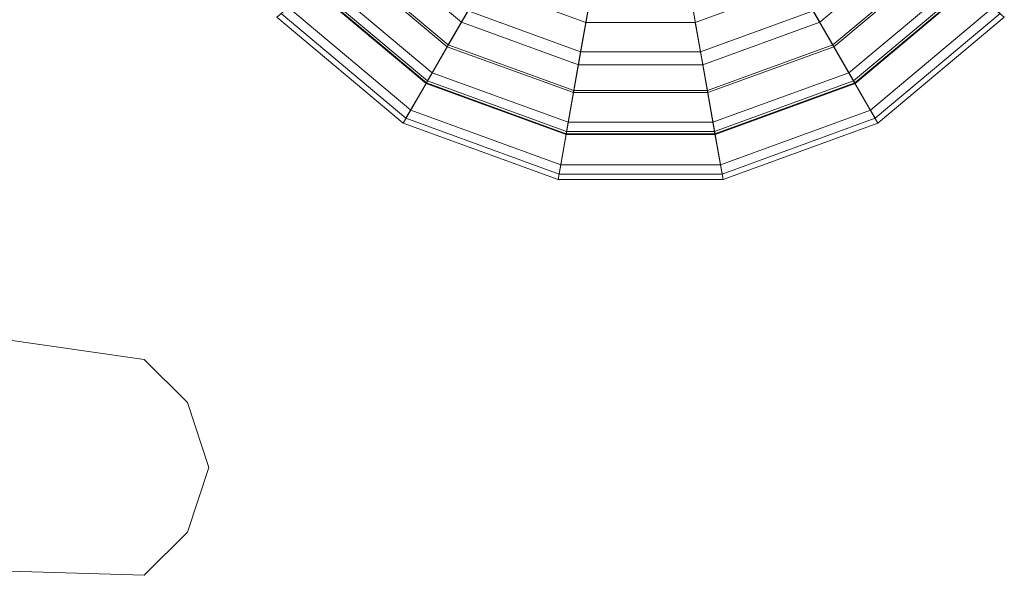
# Model space of a CAD drawing. Units: inches. Extents: x 375 to 1122, y 27 to 1069.
# Tile 20 of 155: x 717.492 to 720.301, y 270.778 to 272.362. Entities that reach past the tile are written whole.
import ezdxf

# ---------------------------------------------------------------- set-up
doc = ezdxf.new("R2010")
doc.units = ezdxf.units.IN
doc.layers.add('Furniture', color=30, linetype='Continuous', lineweight=18)

# ---------------------------------------------------------------- blocks, each defined once
blk = doc.blocks.new('A$C403C54AD')
for points in [[(1.855884, 0.874815, -0.031825), (1.826559, 0.857884, -0.028747), (1.826559, 0.857884, -0.028747), (1.848325, 0.883824, -0.031825)], [(1.853021, 0.873162, 0.131159), (1.855539, 0.874616, 0.117935), (1.848069, 0.883518, 0.117935), (1.8462, 0.881291, 0.131159)], [(1.853056, 0.873182, -0.028594), (1.855884, 0.874815, -0.031825), (1.848325, 0.883824, -0.031825), (1.846226, 0.881322, -0.028594)], [(1.855539, 0.874616, 0.117935), (1.854954, 0.874278, 0.089693), (1.847635, 0.883001, 0.089693), (1.848069, 0.883518, 0.117935)], [(1.854954, 0.874278, 0.089693), (1.850309, 0.871596, 0.071684), (1.844187, 0.878892, 0.071684), (1.847635, 0.883001, 0.089693)], [(1.838869, 0.864991, -0.02532), (1.853056, 0.873182, -0.028594), (1.846226, 0.881322, -0.028594), (1.835696, 0.868773, -0.02532)], [(1.847874, 0.87019, 0.073031), (1.852298, 0.872744, 0.090178), (1.845663, 0.880651, 0.090178), (1.84238, 0.876739, 0.073031)], [(1.848694, 0.870664, 0.140564), (1.853021, 0.873162, 0.131159), (1.8462, 0.881291, 0.131159), (1.842988, 0.877464, 0.140564)], [(1.852868, 0.873073, 0.117718), (1.850434, 0.871669, 0.130354), (1.84428, 0.879003, 0.130354), (1.846086, 0.881156, 0.117718)], [(1.852298, 0.872744, 0.090178), (1.852868, 0.873073, 0.117718), (1.846086, 0.881156, 0.117718), (1.845663, 0.880651, 0.090178)], [(1.850309, 0.871596, 0.071684), (1.844189, 0.868063, 0.061451), (1.839644, 0.873479, 0.061451), (1.844187, 0.878892, 0.071684)], [(1.850434, 0.871669, 0.130354), (1.846028, 0.869125, 0.140564), (1.84101, 0.875106, 0.140564), (1.84428, 0.879003, 0.130354)], [(1.846028, 0.869125, 0.140564), (1.848694, 0.870664, 0.140564), (1.842988, 0.877464, 0.140564), (1.84101, 0.875106, 0.140564)], [(1.859907, 0.863764, -0.031825), (1.826559, 0.857884, -0.028747), (1.826559, 0.857884, -0.028747), (1.855884, 0.874815, -0.031825)], [(1.858849, 0.863578, 0.089693), (1.853566, 0.862646, 0.071684), (1.850309, 0.871596, 0.071684), (1.854954, 0.874278, 0.089693)], [(1.856651, 0.86319, 0.131159), (1.859514, 0.863695, 0.117935), (1.855539, 0.874616, 0.117935), (1.853021, 0.873162, 0.131159)], [(1.85669, 0.863197, -0.028594), (1.859907, 0.863764, -0.031825), (1.855884, 0.874815, -0.031825), (1.853056, 0.873182, -0.028594)], [(1.859514, 0.863695, 0.117935), (1.858849, 0.863578, 0.089693), (1.854954, 0.874278, 0.089693), (1.855539, 0.874616, 0.117935)], [(1.840557, 0.860352, -0.02532), (1.85669, 0.863197, -0.028594), (1.853056, 0.873182, -0.028594), (1.838869, 0.864991, -0.02532)], [(1.85173, 0.862322, 0.140564), (1.856651, 0.86319, 0.131159), (1.853021, 0.873162, 0.131159), (1.848694, 0.870664, 0.140564)], [(1.856476, 0.863159, 0.117718), (1.853709, 0.862671, 0.130354), (1.850434, 0.871669, 0.130354), (1.852868, 0.873073, 0.117718)], [(1.855828, 0.863045, 0.090178), (1.856476, 0.863159, 0.117718), (1.852868, 0.873073, 0.117718), (1.852298, 0.872744, 0.090178)], [(1.850798, 0.862158, 0.073031), (1.855828, 0.863045, 0.090178), (1.852298, 0.872744, 0.090178), (1.847874, 0.87019, 0.073031)], [(1.853566, 0.862646, 0.071684), (1.846607, 0.861419, 0.061451), (1.844189, 0.868063, 0.061451), (1.850309, 0.871596, 0.071684)], [(1.853709, 0.862671, 0.130354), (1.848699, 0.861788, 0.140564), (1.846028, 0.869125, 0.140564), (1.850434, 0.871669, 0.130354)], [(1.844411, 0.861032, 0.063639), (1.850798, 0.862158, 0.073031), (1.847874, 0.87019, 0.073031), (1.842258, 0.866948, 0.063639)], [(1.848699, 0.861788, 0.140564), (1.85173, 0.862322, 0.140564), (1.848694, 0.870664, 0.140564), (1.846028, 0.869125, 0.140564)], [(1.859907, 0.852004, -0.031825), (1.826559, 0.857884, -0.028747), (1.826559, 0.857884, -0.028747), (1.859907, 0.863764, -0.031825)], [(1.85669, 0.852571, -0.028594), (1.859907, 0.852004, -0.031825), (1.859907, 0.863764, -0.031825), (1.85669, 0.863197, -0.028594)], [(1.840557, 0.855416, -0.02532), (1.85669, 0.852571, -0.028594), (1.85669, 0.863197, -0.028594), (1.840557, 0.860352, -0.02532)], [(1.850798, 0.85361, 0.073031), (1.855828, 0.852723, 0.090178), (1.855828, 0.863045, 0.090178), (1.850798, 0.862158, 0.073031)], [(1.85173, 0.853446, 0.140564), (1.856651, 0.852578, 0.131159), (1.856651, 0.86319, 0.131159), (1.85173, 0.862322, 0.140564)], [(1.858849, 0.85219, 0.089693), (1.853566, 0.853122, 0.071684), (1.853566, 0.862646, 0.071684), (1.858849, 0.863578, 0.089693)], [(1.856476, 0.852609, 0.117718), (1.853709, 0.853097, 0.130354), (1.853709, 0.862671, 0.130354), (1.856476, 0.863159, 0.117718)], [(1.855828, 0.852723, 0.090178), (1.856476, 0.852609, 0.117718), (1.856476, 0.863159, 0.117718), (1.855828, 0.863045, 0.090178)], [(1.856651, 0.852578, 0.131159), (1.859514, 0.852073, 0.117935), (1.859514, 0.863695, 0.117935), (1.856651, 0.86319, 0.131159)], [(1.859514, 0.852073, 0.117935), (1.858849, 0.85219, 0.089693), (1.858849, 0.863578, 0.089693), (1.859514, 0.863695, 0.117935)], [(1.853566, 0.853122, 0.071684), (1.846607, 0.854349, 0.061451), (1.846607, 0.861419, 0.061451), (1.853566, 0.862646, 0.071684)], [(1.853709, 0.853097, 0.130354), (1.848699, 0.85398, 0.140564), (1.848699, 0.861788, 0.140564), (1.853709, 0.862671, 0.130354)], [(1.844411, 0.854736, 0.063639), (1.850798, 0.85361, 0.073031), (1.850798, 0.862158, 0.073031), (1.844411, 0.861032, 0.063639)], [(1.848699, 0.85398, 0.140564), (1.85173, 0.853446, 0.140564), (1.85173, 0.862322, 0.140564), (1.848699, 0.861788, 0.140564)], [(1.855884, 0.840953, -0.031825), (1.826559, 0.857884, -0.028747), (1.826559, 0.857884, -0.028747), (1.859907, 0.852004, -0.031825)], [(1.848325, 0.831944, -0.031825), (1.826559, 0.857884, -0.028747), (1.826559, 0.857884, -0.028747), (1.855884, 0.840953, -0.031825)], [(1.838869, 0.850777, -0.02532), (1.853056, 0.842586, -0.028594), (1.85669, 0.852571, -0.028594), (1.840557, 0.855416, -0.02532)], [(1.842258, 0.84882, 0.063639), (1.847874, 0.845577, 0.073031), (1.850798, 0.85361, 0.073031), (1.844411, 0.854736, 0.063639)], [(1.850309, 0.844172, 0.071684), (1.844189, 0.847705, 0.061451), (1.846607, 0.854349, 0.061451), (1.853566, 0.853122, 0.071684)], [(1.846028, 0.846643, 0.140564), (1.848694, 0.845104, 0.140564), (1.85173, 0.853446, 0.140564), (1.848699, 0.85398, 0.140564)], [(1.850434, 0.844099, 0.130354), (1.846028, 0.846643, 0.140564), (1.848699, 0.85398, 0.140564), (1.853709, 0.853097, 0.130354)], [(1.847874, 0.845577, 0.073031), (1.852298, 0.843024, 0.090178), (1.855828, 0.852723, 0.090178), (1.850798, 0.85361, 0.073031)], [(1.848694, 0.845104, 0.140564), (1.853021, 0.842606, 0.131159), (1.856651, 0.852578, 0.131159), (1.85173, 0.853446, 0.140564)], [(1.854954, 0.84149, 0.089693), (1.850309, 0.844172, 0.071684), (1.853566, 0.853122, 0.071684), (1.858849, 0.85219, 0.089693)], [(1.852868, 0.842695, 0.117718), (1.850434, 0.844099, 0.130354), (1.853709, 0.853097, 0.130354), (1.856476, 0.852609, 0.117718)], [(1.852298, 0.843024, 0.090178), (1.852868, 0.842695, 0.117718), (1.856476, 0.852609, 0.117718), (1.855828, 0.852723, 0.090178)], [(1.853021, 0.842606, 0.131159), (1.855539, 0.841152, 0.117935), (1.859514, 0.852073, 0.117935), (1.856651, 0.852578, 0.131159)], [(1.853056, 0.842586, -0.028594), (1.855884, 0.840953, -0.031825), (1.859907, 0.852004, -0.031825), (1.85669, 0.852571, -0.028594)], [(1.855539, 0.841152, 0.117935), (1.854954, 0.84149, 0.089693), (1.858849, 0.85219, 0.089693), (1.859514, 0.852073, 0.117935)], [(1.835696, 0.846995, -0.02532), (1.846226, 0.834446, -0.028594), (1.853056, 0.842586, -0.028594), (1.838869, 0.850777, -0.02532)], [(1.844187, 0.836876, 0.071684), (1.839644, 0.842289, 0.061451), (1.844189, 0.847705, 0.061451), (1.850309, 0.844172, 0.071684)], [(1.84101, 0.840662, 0.140564), (1.842988, 0.838304, 0.140564), (1.848694, 0.845104, 0.140564), (1.846028, 0.846643, 0.140564)], [(1.84428, 0.836765, 0.130354), (1.84101, 0.840662, 0.140564), (1.846028, 0.846643, 0.140564), (1.850434, 0.844099, 0.130354)], [(1.84238, 0.839029, 0.073031), (1.845663, 0.835117, 0.090178), (1.852298, 0.843024, 0.090178), (1.847874, 0.845577, 0.073031)], [(1.842988, 0.838304, 0.140564), (1.8462, 0.834477, 0.131159), (1.853021, 0.842606, 0.131159), (1.848694, 0.845104, 0.140564)], [(1.847635, 0.832767, 0.089693), (1.844187, 0.836876, 0.071684), (1.850309, 0.844172, 0.071684), (1.854954, 0.84149, 0.089693)], [(1.846086, 0.834612, 0.117718), (1.84428, 0.836765, 0.130354), (1.850434, 0.844099, 0.130354), (1.852868, 0.842695, 0.117718)], [(1.845663, 0.835117, 0.090178), (1.846086, 0.834612, 0.117718), (1.852868, 0.842695, 0.117718), (1.852298, 0.843024, 0.090178)], [(1.8462, 0.834477, 0.131159), (1.848069, 0.83225, 0.117935), (1.855539, 0.841152, 0.117935), (1.853021, 0.842606, 0.131159)], [(1.846226, 0.834446, -0.028594), (1.848325, 0.831944, -0.031825), (1.855884, 0.840953, -0.031825), (1.853056, 0.842586, -0.028594)], [(1.848069, 0.83225, 0.117935), (1.847635, 0.832767, 0.089693), (1.854954, 0.84149, 0.089693), (1.855539, 0.841152, 0.117935)]]:
    blk.add_3dface(points)
for points, invisible_edges in [([(1.880431, 0.8271, -0.024899), (1.880431, 0.8271, -0.024899), (1.885048, 0.825561, -0.024899), (1.875813, 0.825561, -0.024899)], 4), ([(1.880431, 0.8271, -0.026438), (1.880431, 0.8271, -0.026438), (1.885048, 0.825561, -0.026438), (1.875813, 0.825561, -0.026438)], 4), ([(1.880431, 0.8271, -0.024899), (1.880431, 0.8271, -0.026438), (1.875813, 0.825561, -0.026438), (1.875813, 0.825561, -0.024899)], 4), ([(1.885048, 0.825561, -0.026438), (1.885048, 0.825561, -0.024899), (1.880431, 0.8271, -0.024899), (1.880431, 0.8271, -0.026438)], 1), ([(1.885048, 0.825561, -0.024899), (1.875813, 0.825561, -0.024899), (1.872735, 0.822483, -0.024899), (1.888127, 0.822483, -0.024899)], 5), ([(1.885048, 0.825561, -0.026438), (1.875813, 0.825561, -0.026438), (1.872735, 0.822483, -0.026438), (1.888127, 0.822483, -0.026438)], 5), ([(1.875813, 0.825561, -0.026438), (1.875813, 0.825561, -0.024899), (1.872735, 0.822483, -0.024899), (1.872735, 0.822483, -0.026438)], 5), ([(1.888127, 0.822483, -0.024899), (1.888127, 0.822483, -0.026438), (1.885048, 0.825561, -0.026438), (1.885048, 0.825561, -0.024899)], 5), ([(1.872735, 0.822483, -0.024899), (1.888127, 0.822483, -0.024899), (1.886587, 0.773228, -0.024899), (1.871195, 0.811708, -0.024899)], 5), ([(1.872735, 0.822483, -0.026438), (1.888127, 0.822483, -0.026438), (1.886587, 0.773228, -0.026438), (1.871195, 0.811708, -0.026438)], 5), ([(1.872735, 0.822483, -0.024899), (1.872735, 0.822483, -0.026438), (1.871195, 0.811708, -0.026438), (1.871195, 0.811708, -0.024899)], 5), ([(1.886587, 0.773228, -0.026438), (1.886587, 0.773228, -0.024899), (1.888127, 0.822483, -0.024899), (1.888127, 0.822483, -0.026438)], 5)]:
    blk.add_3dface(points, dxfattribs=dict(invisible_edges=invisible_edges))

msp = doc.modelspace()

# ---------------------------------------------------------------- block references
at = {"layer": 'Furniture', "xscale": 39.9918517141215, "yscale": 39.9918517141215, "zscale": 39.9918517141215, "rotation": 270}
msp.add_blockref('A$C403C54AD', (684.9549, 346.2875, 0.024), dxfattribs=at)

doc.saveas('drawing.dxf')
